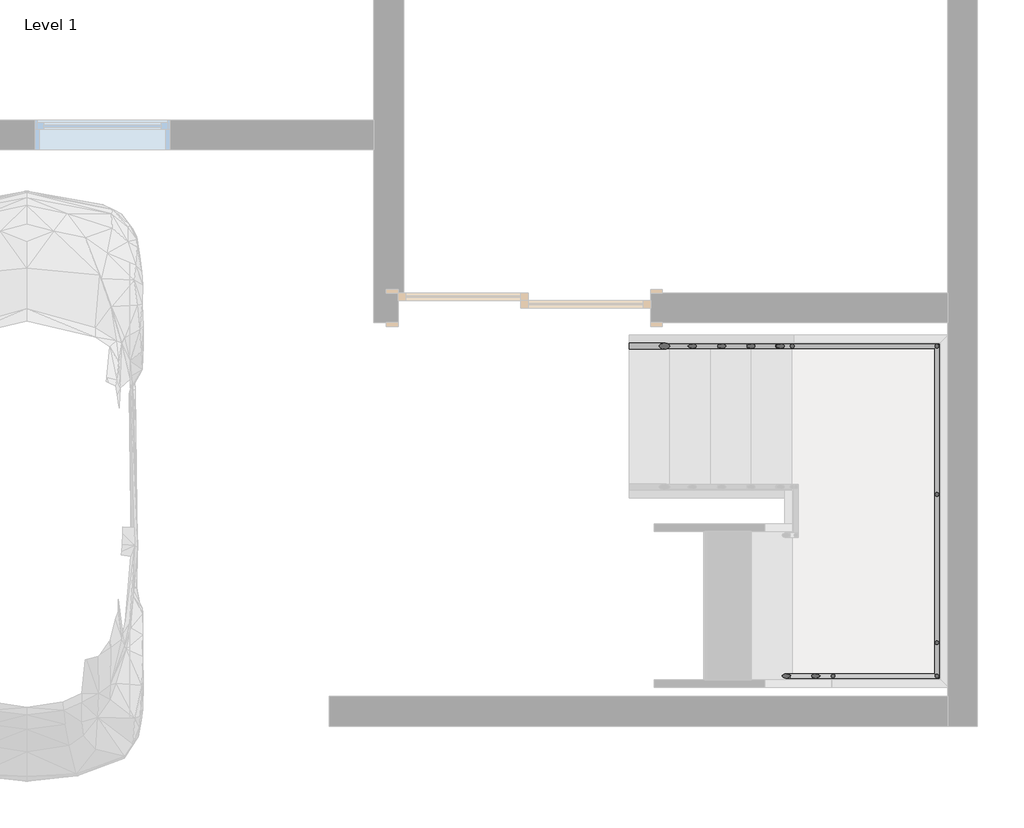
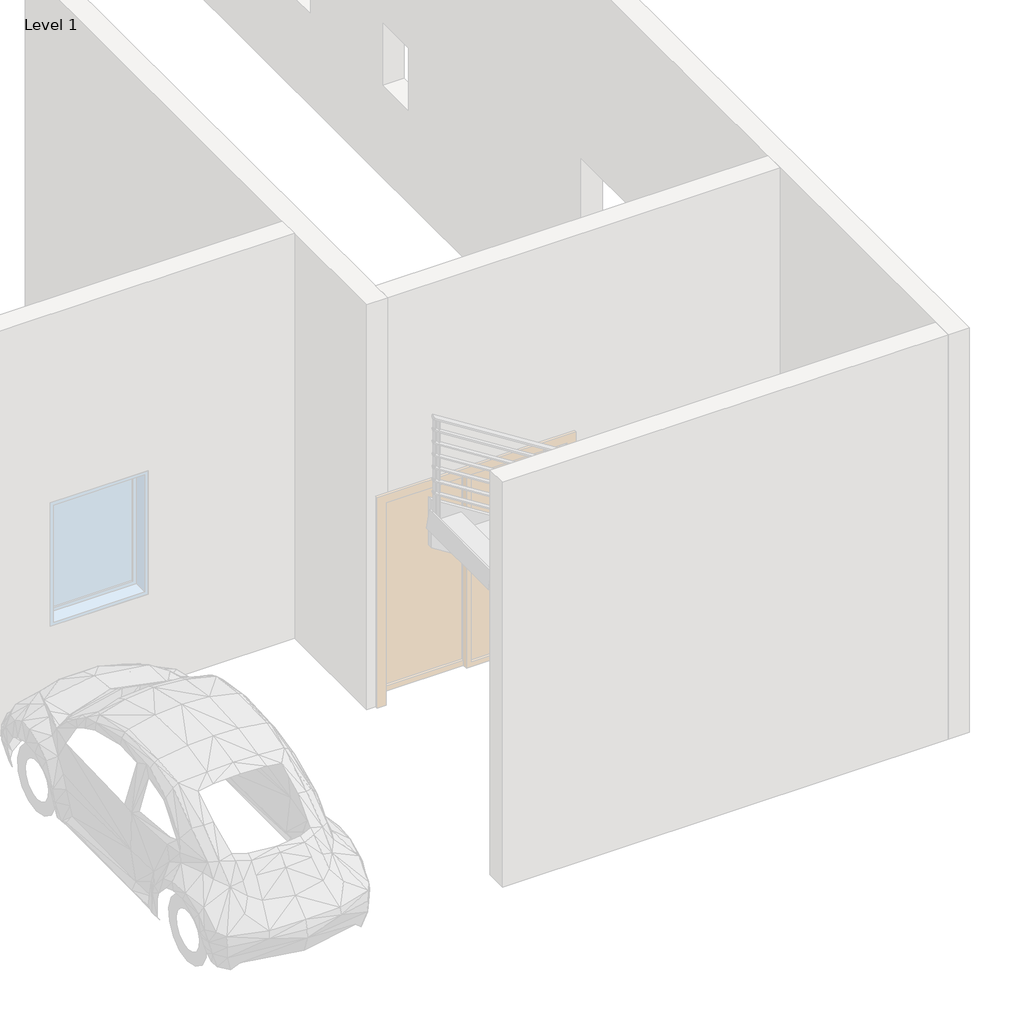
# One storey, part 3 of 4: 1 railing.
"""IFC4 building model written with IfcOpenShell, lengths in millimetres."""

from ifc_helpers import new_model, si_unit, point, frame, frame_2d, origin, place, context, project, spatial, circle_curve, ellipse_curve, trimmed, segment, composite_curve, outline, extrude, element, save
from ifc_brep_helpers import plane_surface, cylinder_surface, advanced_brep

model = new_model("IFC4")

# Units and contexts
model_context = context("Model", 3, world=origin())
ifc_project = project(units=[si_unit("LENGTHUNIT", "METRE", prefix="MILLI")], contexts=[model_context])

# Site, building, storey
site = spatial("IfcSite", under=ifc_project)
building = spatial("IfcBuilding", under=site)
storey = spatial("IfcBuildingStorey", under=building, Name="Level 1", Elevation=0.0)

# Railing
placement = place(None, origin())
element("IfcRailing", 1, ObjectType="900mm Pipe", at=placement, inside=storey, context=model_context, shape_type="SolidModel", body=[
    advanced_brep(
    [(-3791.9701746, -1586.5632824, 1050.2491997), (-3791.9701746, -1546.5632824, 1050.2491997), (-2686.1767216, -1586.5632824, 1749.5652174), (-2686.1767216, -1546.5632824, 1749.5652174), (-1737.3443934, -1586.5632824, 1749.5652174), (-1697.3443934, -1546.5632824, 1749.5652174), (-1737.3443934, -3770.8148449, 1749.5652174), (-1697.3443934, -3810.8148449, 1749.5652174), (-2422.7636276, -3770.8148449, 1749.5652174), (-2422.7636276, -3810.8148449, 1749.5652174), (-5716.9701746, -3770.8148449, 3832.8578953), (-5716.9701746, -3810.8148449, 3832.8578953)],
    [
        (0, 1, ellipse_curve(frame((-3791.9701746, -1566.5632824, 1050.2491997), z_axis=(-1.0, 0.0, 0.0), x_axis=(0.0, 0.0, -1.0)), 23.6638438, 20.0)),
        (1, 0, ellipse_curve(frame((-3791.9701746, -1566.5632824, 1050.2491997), z_axis=(-1.0, 0.0, 0.0), x_axis=(0.0, 0.0, -1.0)), 23.6638438, 20.0)),
        (0, 2),
        (2, 3, ellipse_curve(frame((-2686.1767216, -1566.5632824, 1749.5652174), z_axis=(-0.9605132043335073, 0.0, -0.27823440531497545), x_axis=(0.27823440531497523, 0.0, -0.9605132043335074)), 20.822202, 20.0)),
        (3, 1),
        (3, 2, ellipse_curve(frame((-2686.1767216, -1566.5632824, 1749.5652174), z_axis=(-0.9605132043335073, 0.0, -0.27823440531497545), x_axis=(0.27823440531497523, 0.0, -0.9605132043335074)), 20.822202, 20.0)),
        (2, 4),
        (4, 5, ellipse_curve(frame((-1717.3443934, -1566.5632824, 1749.5652174), z_axis=(-0.7071067811865449, 0.70710678118655, 0.0), x_axis=(-0.7071067811865501, -0.7071067811865448, 0.0)), 28.2842712, 20.0)),
        (5, 3),
        (5, 4, ellipse_curve(frame((-1717.3443934, -1566.5632824, 1749.5652174), z_axis=(-0.7071067811865449, 0.70710678118655, 0.0), x_axis=(-0.7071067811865501, -0.7071067811865448, 0.0)), 28.2842712, 20.0)),
        (4, 6),
        (6, 7, ellipse_curve(frame((-1717.3443934, -3790.8148449, 1749.5652174), z_axis=(0.70710678118655, 0.7071067811865449, 0.0), x_axis=(-0.7071067811865448, 0.7071067811865502, 0.0)), 28.2842712, 20.0)),
        (7, 5),
        (7, 6, ellipse_curve(frame((-1717.3443934, -3790.8148449, 1749.5652174), z_axis=(0.70710678118655, 0.7071067811865449, 0.0), x_axis=(-0.7071067811865448, 0.7071067811865502, 0.0)), 28.2842712, 20.0)),
        (6, 8),
        (8, 9, ellipse_curve(frame((-2422.7636276, -3790.8148449, 1749.5652174), z_axis=(0.9605132043335072, 0.0, -0.27823440531497556), x_axis=(0.27823440531497595, 0.0, 0.9605132043335071)), 20.822202, 20.0)),
        (9, 7),
        (9, 8, ellipse_curve(frame((-2422.7636276, -3790.8148449, 1749.5652174), z_axis=(0.9605132043335072, 0.0, -0.27823440531497556), x_axis=(0.27823440531497595, 0.0, 0.9605132043335071)), 20.822202, 20.0)),
        (10, 11, ellipse_curve(frame((-5716.9701746, -3790.8148449, 3832.8578953), z_axis=(-1.0, 0.0, 0.0), x_axis=(0.0, 0.0, -1.0)), 23.6638438, 20.0)),
        (11, 10, ellipse_curve(frame((-5716.9701746, -3790.8148449, 3832.8578953), z_axis=(-1.0, 0.0, 0.0), x_axis=(0.0, 0.0, -1.0)), 23.6638438, 20.0)),
        (8, 10),
        (11, 9),
    ],
    [
        plane_surface(frame((-3791.9701746, -1566.5632824, 1073.9130435), z_axis=(-1.0, 0.0, 0.0), x_axis=(0.0, 1.0, 0.0))),
        cylinder_surface(frame((-3781.2802618, -1566.5632824, 1057.0096189), z_axis=(-0.8451712313980438, 0.0, -0.53449564040983), x_axis=(0.0, 1.0, 0.0)), 20.0),
        cylinder_surface(frame((-2691.9701746, -1566.5632824, 1749.5652174), z_axis=(-1.0, 0.0, 0.0), x_axis=(0.0, 1.0, 0.0)), 20.0),
        cylinder_surface(frame((-1717.3443934, -1566.5632824, 1749.5652174), z_axis=(0.0, 1.0, 0.0), x_axis=(1.0, 0.0, 0.0)), 20.0),
        cylinder_surface(frame((-1717.3443934, -3790.8148449, 1749.5652174), z_axis=(1.0, 0.0, 0.0), x_axis=(0.0, -1.0, 0.0)), 20.0),
        plane_surface(frame((-5716.9701746, -3790.8148449, 3856.5217391), z_axis=(-1.0, 0.0, 0.0), x_axis=(0.0, -1.0, 0.0))),
        cylinder_surface(frame((-2427.6600875, -3790.8148449, 1752.6617928), z_axis=(0.8451712313980437, 0.0, -0.5344956404098302), x_axis=(0.0, -1.0, 0.0)), 20.0),
    ],
    [
        (0, [[1, 2]]),
        (1, [[-1, 3, 4, 5]]),
        (1, [[-2, -5, 6, -3]]),
        (2, [[-4, 7, 8, 9]]),
        (2, [[-6, -9, 10, -7]]),
        (3, [[-8, 11, 12, 13]]),
        (3, [[-10, -13, 14, -11]]),
        (4, [[-12, 15, 16, 17]]),
        (4, [[-14, -17, 18, -15]]),
        (5, [[19, 20]]),
        (6, [[-16, 21, -20, 22]]),
        (6, [[-18, -22, -19, -21]]),
    ],
),
    advanced_brep(
    [(-3791.9701746, -1581.5632824, 931.1651606), (-3791.9701746, -1551.5632824, 931.1651606), (-2687.6250849, -1581.5632824, 1629.5652174), (-2687.6250849, -1551.5632824, 1629.5652174), (-1732.3443934, -1581.5632824, 1629.5652174), (-1702.3443934, -1551.5632824, 1629.5652174), (-1732.3443934, -3775.8148449, 1629.5652174), (-1702.3443934, -3805.8148449, 1629.5652174), (-2421.3152644, -3775.8148449, 1629.5652174), (-2421.3152644, -3805.8148449, 1629.5652174), (-5716.9701746, -3775.8148449, 3713.7738563), (-5716.9701746, -3805.8148449, 3713.7738563)],
    [
        (0, 1, ellipse_curve(frame((-3791.9701746, -1566.5632824, 931.1651606), z_axis=(-1.0, 0.0, 0.0), x_axis=(0.0, 0.0, -1.0)), 17.7478828, 15.0)),
        (1, 0, ellipse_curve(frame((-3791.9701746, -1566.5632824, 931.1651606), z_axis=(-1.0, 0.0, 0.0), x_axis=(0.0, 0.0, -1.0)), 17.7478828, 15.0)),
        (0, 2),
        (2, 3, ellipse_curve(frame((-2687.6250849, -1566.5632824, 1629.5652174), z_axis=(-0.9605132043335073, 0.0, -0.27823440531497545), x_axis=(0.2782344053149749, 0.0, -0.9605132043335074)), 15.6166515, 15.0)),
        (3, 1),
        (3, 2, ellipse_curve(frame((-2687.6250849, -1566.5632824, 1629.5652174), z_axis=(-0.9605132043335073, 0.0, -0.27823440531497545), x_axis=(0.2782344053149749, 0.0, -0.9605132043335074)), 15.6166515, 15.0)),
        (2, 4),
        (4, 5, ellipse_curve(frame((-1717.3443934, -1566.5632824, 1629.5652174), z_axis=(-0.7071067811865449, 0.70710678118655, 0.0), x_axis=(-0.7071067811865501, -0.7071067811865448, 0.0)), 21.2132034, 15.0)),
        (5, 3),
        (5, 4, ellipse_curve(frame((-1717.3443934, -1566.5632824, 1629.5652174), z_axis=(-0.7071067811865449, 0.70710678118655, 0.0), x_axis=(-0.7071067811865501, -0.7071067811865448, 0.0)), 21.2132034, 15.0)),
        (4, 6),
        (6, 7, ellipse_curve(frame((-1717.3443934, -3790.8148449, 1629.5652174), z_axis=(0.70710678118655, 0.7071067811865449, 0.0), x_axis=(-0.7071067811865448, 0.7071067811865502, 0.0)), 21.2132034, 15.0)),
        (7, 5),
        (7, 6, ellipse_curve(frame((-1717.3443934, -3790.8148449, 1629.5652174), z_axis=(0.70710678118655, 0.7071067811865449, 0.0), x_axis=(-0.7071067811865448, 0.7071067811865502, 0.0)), 21.2132034, 15.0)),
        (6, 8),
        (8, 9, ellipse_curve(frame((-2421.3152644, -3790.8148449, 1629.5652174), z_axis=(0.9605132043335072, 0.0, -0.2782344053149756), x_axis=(0.27823440531497595, 0.0, 0.9605132043335071)), 15.6166515, 15.0)),
        (9, 7),
        (9, 8, ellipse_curve(frame((-2421.3152644, -3790.8148449, 1629.5652174), z_axis=(0.9605132043335072, 0.0, -0.2782344053149756), x_axis=(0.27823440531497595, 0.0, 0.9605132043335071)), 15.6166515, 15.0)),
        (10, 11, ellipse_curve(frame((-5716.9701746, -3790.8148449, 3713.7738563), z_axis=(-1.0, 0.0, 0.0), x_axis=(0.0, 0.0, -1.0)), 17.7478828, 15.0)),
        (11, 10, ellipse_curve(frame((-5716.9701746, -3790.8148449, 3713.7738563), z_axis=(-1.0, 0.0, 0.0), x_axis=(0.0, 0.0, -1.0)), 17.7478828, 15.0)),
        (8, 10),
        (11, 9),
    ],
    [
        plane_surface(frame((-3791.9701746, -1566.5632824, 948.9130435), z_axis=(-1.0, 0.0, 0.0), x_axis=(0.0, 1.0, 0.0))),
        cylinder_surface(frame((-3783.95274, -1566.5632824, 936.235475), z_axis=(-0.845171231398044, 0.0, -0.5344956404098299), x_axis=(0.0, 1.0, 0.0)), 15.0),
        cylinder_surface(frame((-2691.9701746, -1566.5632824, 1629.5652174), z_axis=(-1.0, 0.0, 0.0), x_axis=(0.0, 1.0, 0.0)), 15.0),
        cylinder_surface(frame((-1717.3443934, -1566.5632824, 1629.5652174), z_axis=(0.0, 1.0, 0.0), x_axis=(1.0, 0.0, 0.0)), 15.0),
        cylinder_surface(frame((-1717.3443934, -3790.8148449, 1629.5652174), z_axis=(1.0, 0.0, 0.0), x_axis=(0.0, -1.0, 0.0)), 15.0),
        plane_surface(frame((-5716.9701746, -3790.8148449, 3731.5217391), z_axis=(-1.0, 0.0, 0.0), x_axis=(0.0, -1.0, 0.0))),
        cylinder_surface(frame((-2424.9876092, -3790.8148449, 1631.8876489), z_axis=(0.8451712313980437, 0.0, -0.5344956404098302), x_axis=(0.0, -1.0, 0.0)), 15.0),
    ],
    [
        (0, [[1, 2]]),
        (1, [[-1, 3, 4, 5]]),
        (1, [[-2, -5, 6, -3]]),
        (2, [[-4, 7, 8, 9]]),
        (2, [[-6, -9, 10, -7]]),
        (3, [[-8, 11, 12, 13]]),
        (3, [[-10, -13, 14, -11]]),
        (4, [[-12, 15, 16, 17]]),
        (4, [[-14, -17, 18, -15]]),
        (5, [[19, 20]]),
        (6, [[-16, 21, -20, 22]]),
        (6, [[-18, -22, -19, -21]]),
    ],
),
    advanced_brep(
    [(-3791.9701746, -1581.5632824, 806.1651606), (-3791.9701746, -1551.5632824, 806.1651606), (-2687.6250849, -1581.5632824, 1504.5652174), (-2687.6250849, -1551.5632824, 1504.5652174), (-1732.3443934, -1581.5632824, 1504.5652174), (-1702.3443934, -1551.5632824, 1504.5652174), (-1732.3443934, -3775.8148449, 1504.5652174), (-1702.3443934, -3805.8148449, 1504.5652174), (-2421.3152644, -3775.8148449, 1504.5652174), (-2421.3152644, -3805.8148449, 1504.5652174), (-5716.9701746, -3775.8148449, 3588.7738563), (-5716.9701746, -3805.8148449, 3588.7738563)],
    [
        (0, 1, ellipse_curve(frame((-3791.9701746, -1566.5632824, 806.1651606), z_axis=(-1.0, 0.0, 0.0), x_axis=(0.0, 0.0, -1.0)), 17.7478828, 15.0)),
        (1, 0, ellipse_curve(frame((-3791.9701746, -1566.5632824, 806.1651606), z_axis=(-1.0, 0.0, 0.0), x_axis=(0.0, 0.0, -1.0)), 17.7478828, 15.0)),
        (0, 2),
        (2, 3, ellipse_curve(frame((-2687.6250849, -1566.5632824, 1504.5652174), z_axis=(-0.9605132043335073, 0.0, -0.27823440531497545), x_axis=(0.2782344053149749, 0.0, -0.9605132043335074)), 15.6166515, 15.0)),
        (3, 1),
        (3, 2, ellipse_curve(frame((-2687.6250849, -1566.5632824, 1504.5652174), z_axis=(-0.9605132043335073, 0.0, -0.27823440531497545), x_axis=(0.2782344053149749, 0.0, -0.9605132043335074)), 15.6166515, 15.0)),
        (2, 4),
        (4, 5, ellipse_curve(frame((-1717.3443934, -1566.5632824, 1504.5652174), z_axis=(-0.7071067811865449, 0.70710678118655, 0.0), x_axis=(-0.7071067811865501, -0.7071067811865448, 0.0)), 21.2132034, 15.0)),
        (5, 3),
        (5, 4, ellipse_curve(frame((-1717.3443934, -1566.5632824, 1504.5652174), z_axis=(-0.7071067811865449, 0.70710678118655, 0.0), x_axis=(-0.7071067811865501, -0.7071067811865448, 0.0)), 21.2132034, 15.0)),
        (4, 6),
        (6, 7, ellipse_curve(frame((-1717.3443934, -3790.8148449, 1504.5652174), z_axis=(0.70710678118655, 0.7071067811865449, 0.0), x_axis=(-0.7071067811865448, 0.7071067811865502, 0.0)), 21.2132034, 15.0)),
        (7, 5),
        (7, 6, ellipse_curve(frame((-1717.3443934, -3790.8148449, 1504.5652174), z_axis=(0.70710678118655, 0.7071067811865449, 0.0), x_axis=(-0.7071067811865448, 0.7071067811865502, 0.0)), 21.2132034, 15.0)),
        (6, 8),
        (8, 9, ellipse_curve(frame((-2421.3152644, -3790.8148449, 1504.5652174), z_axis=(0.9605132043335072, 0.0, -0.2782344053149756), x_axis=(0.27823440531497595, 0.0, 0.9605132043335071)), 15.6166515, 15.0)),
        (9, 7),
        (9, 8, ellipse_curve(frame((-2421.3152644, -3790.8148449, 1504.5652174), z_axis=(0.9605132043335072, 0.0, -0.2782344053149756), x_axis=(0.27823440531497595, 0.0, 0.9605132043335071)), 15.6166515, 15.0)),
        (10, 11, ellipse_curve(frame((-5716.9701746, -3790.8148449, 3588.7738563), z_axis=(-1.0, 0.0, 0.0), x_axis=(0.0, 0.0, -1.0)), 17.7478828, 15.0)),
        (11, 10, ellipse_curve(frame((-5716.9701746, -3790.8148449, 3588.7738563), z_axis=(-1.0, 0.0, 0.0), x_axis=(0.0, 0.0, -1.0)), 17.7478828, 15.0)),
        (8, 10),
        (11, 9),
    ],
    [
        plane_surface(frame((-3791.9701746, -1566.5632824, 823.9130435), z_axis=(-1.0, 0.0, 0.0), x_axis=(0.0, 1.0, 0.0))),
        cylinder_surface(frame((-3783.95274, -1566.5632824, 811.235475), z_axis=(-0.845171231398044, 0.0, -0.5344956404098299), x_axis=(0.0, 1.0, 0.0)), 15.0),
        cylinder_surface(frame((-2691.9701746, -1566.5632824, 1504.5652174), z_axis=(-1.0, 0.0, 0.0), x_axis=(0.0, 1.0, 0.0)), 15.0),
        cylinder_surface(frame((-1717.3443934, -1566.5632824, 1504.5652174), z_axis=(0.0, 1.0, 0.0), x_axis=(1.0, 0.0, 0.0)), 15.0),
        cylinder_surface(frame((-1717.3443934, -3790.8148449, 1504.5652174), z_axis=(1.0, 0.0, 0.0), x_axis=(0.0, -1.0, 0.0)), 15.0),
        plane_surface(frame((-5716.9701746, -3790.8148449, 3606.5217391), z_axis=(-1.0, 0.0, 0.0), x_axis=(0.0, -1.0, 0.0))),
        cylinder_surface(frame((-2424.9876092, -3790.8148449, 1506.8876489), z_axis=(0.8451712313980437, 0.0, -0.5344956404098302), x_axis=(0.0, -1.0, 0.0)), 15.0),
    ],
    [
        (0, [[1, 2]]),
        (1, [[-1, 3, 4, 5]]),
        (1, [[-2, -5, 6, -3]]),
        (2, [[-4, 7, 8, 9]]),
        (2, [[-6, -9, 10, -7]]),
        (3, [[-8, 11, 12, 13]]),
        (3, [[-10, -13, 14, -11]]),
        (4, [[-12, 15, 16, 17]]),
        (4, [[-14, -17, 18, -15]]),
        (5, [[19, 20]]),
        (6, [[-16, 21, -20, 22]]),
        (6, [[-18, -22, -19, -21]]),
    ],
),
    advanced_brep(
    [(-3791.9701746, -1581.5632824, 681.1651606), (-3791.9701746, -1551.5632824, 681.1651606), (-2687.6250849, -1581.5632824, 1379.5652174), (-2687.6250849, -1551.5632824, 1379.5652174), (-1732.3443934, -1581.5632824, 1379.5652174), (-1702.3443934, -1551.5632824, 1379.5652174), (-1732.3443934, -3775.8148449, 1379.5652174), (-1702.3443934, -3805.8148449, 1379.5652174), (-2421.3152644, -3775.8148449, 1379.5652174), (-2421.3152644, -3805.8148449, 1379.5652174), (-5716.9701746, -3775.8148449, 3463.7738563), (-5716.9701746, -3805.8148449, 3463.7738563)],
    [
        (0, 1, ellipse_curve(frame((-3791.9701746, -1566.5632824, 681.1651606), z_axis=(-1.0, 0.0, 0.0), x_axis=(0.0, 0.0, -1.0)), 17.7478828, 15.0)),
        (1, 0, ellipse_curve(frame((-3791.9701746, -1566.5632824, 681.1651606), z_axis=(-1.0, 0.0, 0.0), x_axis=(0.0, 0.0, -1.0)), 17.7478828, 15.0)),
        (0, 2),
        (2, 3, ellipse_curve(frame((-2687.6250849, -1566.5632824, 1379.5652174), z_axis=(-0.9605132043335073, 0.0, -0.27823440531497545), x_axis=(0.2782344053149749, 0.0, -0.9605132043335074)), 15.6166515, 15.0)),
        (3, 1),
        (3, 2, ellipse_curve(frame((-2687.6250849, -1566.5632824, 1379.5652174), z_axis=(-0.9605132043335073, 0.0, -0.27823440531497545), x_axis=(0.2782344053149749, 0.0, -0.9605132043335074)), 15.6166515, 15.0)),
        (2, 4),
        (4, 5, ellipse_curve(frame((-1717.3443934, -1566.5632824, 1379.5652174), z_axis=(-0.7071067811865449, 0.70710678118655, 0.0), x_axis=(-0.7071067811865501, -0.7071067811865448, 0.0)), 21.2132034, 15.0)),
        (5, 3),
        (5, 4, ellipse_curve(frame((-1717.3443934, -1566.5632824, 1379.5652174), z_axis=(-0.7071067811865449, 0.70710678118655, 0.0), x_axis=(-0.7071067811865501, -0.7071067811865448, 0.0)), 21.2132034, 15.0)),
        (4, 6),
        (6, 7, ellipse_curve(frame((-1717.3443934, -3790.8148449, 1379.5652174), z_axis=(0.70710678118655, 0.7071067811865449, 0.0), x_axis=(-0.7071067811865448, 0.7071067811865502, 0.0)), 21.2132034, 15.0)),
        (7, 5),
        (7, 6, ellipse_curve(frame((-1717.3443934, -3790.8148449, 1379.5652174), z_axis=(0.70710678118655, 0.7071067811865449, 0.0), x_axis=(-0.7071067811865448, 0.7071067811865502, 0.0)), 21.2132034, 15.0)),
        (6, 8),
        (8, 9, ellipse_curve(frame((-2421.3152644, -3790.8148449, 1379.5652174), z_axis=(0.9605132043335072, 0.0, -0.27823440531497556), x_axis=(0.27823440531497606, 0.0, 0.9605132043335073)), 15.6166515, 15.0)),
        (9, 7),
        (9, 8, ellipse_curve(frame((-2421.3152644, -3790.8148449, 1379.5652174), z_axis=(0.9605132043335072, 0.0, -0.27823440531497556), x_axis=(0.27823440531497606, 0.0, 0.9605132043335073)), 15.6166515, 15.0)),
        (10, 11, ellipse_curve(frame((-5716.9701746, -3790.8148449, 3463.7738563), z_axis=(-1.0, 0.0, 0.0), x_axis=(0.0, 0.0, -1.0)), 17.7478828, 15.0)),
        (11, 10, ellipse_curve(frame((-5716.9701746, -3790.8148449, 3463.7738563), z_axis=(-1.0, 0.0, 0.0), x_axis=(0.0, 0.0, -1.0)), 17.7478828, 15.0)),
        (8, 10),
        (11, 9),
    ],
    [
        plane_surface(frame((-3791.9701746, -1566.5632824, 698.9130435), z_axis=(-1.0, 0.0, 0.0), x_axis=(0.0, 1.0, 0.0))),
        cylinder_surface(frame((-3783.95274, -1566.5632824, 686.235475), z_axis=(-0.845171231398044, 0.0, -0.5344956404098299), x_axis=(0.0, 1.0, 0.0)), 15.0),
        cylinder_surface(frame((-2691.9701746, -1566.5632824, 1379.5652174), z_axis=(-1.0, 0.0, 0.0), x_axis=(0.0, 1.0, 0.0)), 15.0),
        cylinder_surface(frame((-1717.3443934, -1566.5632824, 1379.5652174), z_axis=(0.0, 1.0, 0.0), x_axis=(1.0, 0.0, 0.0)), 15.0),
        cylinder_surface(frame((-1717.3443934, -3790.8148449, 1379.5652174), z_axis=(1.0, 0.0, 0.0), x_axis=(0.0, -1.0, 0.0)), 15.0),
        plane_surface(frame((-5716.9701746, -3790.8148449, 3481.5217391), z_axis=(-1.0, 0.0, 0.0), x_axis=(0.0, -1.0, 0.0))),
        cylinder_surface(frame((-2424.9876092, -3790.8148449, 1381.8876489), z_axis=(0.8451712313980437, 0.0, -0.5344956404098301), x_axis=(0.0, -1.0, 0.0)), 15.0),
    ],
    [
        (0, [[1, 2]]),
        (1, [[-1, 3, 4, 5]]),
        (1, [[-2, -5, 6, -3]]),
        (2, [[-4, 7, 8, 9]]),
        (2, [[-6, -9, 10, -7]]),
        (3, [[-8, 11, 12, 13]]),
        (3, [[-10, -13, 14, -11]]),
        (4, [[-12, 15, 16, 17]]),
        (4, [[-14, -17, 18, -15]]),
        (5, [[19, 20]]),
        (6, [[-16, 21, -20, 22]]),
        (6, [[-18, -22, -19, -21]]),
    ],
),
    advanced_brep(
    [(-3791.9701746, -1581.5632824, 556.1651606), (-3791.9701746, -1551.5632824, 556.1651606), (-2687.6250849, -1581.5632824, 1254.5652174), (-2687.6250849, -1551.5632824, 1254.5652174), (-1732.3443934, -1581.5632824, 1254.5652174), (-1702.3443934, -1551.5632824, 1254.5652174), (-1732.3443934, -3775.8148449, 1254.5652174), (-1702.3443934, -3805.8148449, 1254.5652174), (-2421.3152644, -3775.8148449, 1254.5652174), (-2421.3152644, -3805.8148449, 1254.5652174), (-5716.9701746, -3775.8148449, 3338.7738563), (-5716.9701746, -3805.8148449, 3338.7738563)],
    [
        (0, 1, ellipse_curve(frame((-3791.9701746, -1566.5632824, 556.1651606), z_axis=(-1.0, 0.0, 0.0), x_axis=(0.0, 0.0, -1.0)), 17.7478828, 15.0)),
        (1, 0, ellipse_curve(frame((-3791.9701746, -1566.5632824, 556.1651606), z_axis=(-1.0, 0.0, 0.0), x_axis=(0.0, 0.0, -1.0)), 17.7478828, 15.0)),
        (0, 2),
        (2, 3, ellipse_curve(frame((-2687.6250849, -1566.5632824, 1254.5652174), z_axis=(-0.9605132043335073, 0.0, -0.27823440531497545), x_axis=(0.2782344053149749, 0.0, -0.9605132043335074)), 15.6166515, 15.0)),
        (3, 1),
        (3, 2, ellipse_curve(frame((-2687.6250849, -1566.5632824, 1254.5652174), z_axis=(-0.9605132043335073, 0.0, -0.27823440531497545), x_axis=(0.2782344053149749, 0.0, -0.9605132043335074)), 15.6166515, 15.0)),
        (2, 4),
        (4, 5, ellipse_curve(frame((-1717.3443934, -1566.5632824, 1254.5652174), z_axis=(-0.7071067811865449, 0.70710678118655, 0.0), x_axis=(-0.7071067811865501, -0.7071067811865448, 0.0)), 21.2132034, 15.0)),
        (5, 3),
        (5, 4, ellipse_curve(frame((-1717.3443934, -1566.5632824, 1254.5652174), z_axis=(-0.7071067811865449, 0.70710678118655, 0.0), x_axis=(-0.7071067811865501, -0.7071067811865448, 0.0)), 21.2132034, 15.0)),
        (4, 6),
        (6, 7, ellipse_curve(frame((-1717.3443934, -3790.8148449, 1254.5652174), z_axis=(0.70710678118655, 0.7071067811865449, 0.0), x_axis=(-0.7071067811865448, 0.7071067811865502, 0.0)), 21.2132034, 15.0)),
        (7, 5),
        (7, 6, ellipse_curve(frame((-1717.3443934, -3790.8148449, 1254.5652174), z_axis=(0.70710678118655, 0.7071067811865449, 0.0), x_axis=(-0.7071067811865448, 0.7071067811865502, 0.0)), 21.2132034, 15.0)),
        (6, 8),
        (8, 9, ellipse_curve(frame((-2421.3152644, -3790.8148449, 1254.5652174), z_axis=(0.9605132043335072, 0.0, -0.2782344053149756), x_axis=(0.27823440531497595, 0.0, 0.9605132043335071)), 15.6166515, 15.0)),
        (9, 7),
        (9, 8, ellipse_curve(frame((-2421.3152644, -3790.8148449, 1254.5652174), z_axis=(0.9605132043335072, 0.0, -0.2782344053149756), x_axis=(0.27823440531497595, 0.0, 0.9605132043335071)), 15.6166515, 15.0)),
        (10, 11, ellipse_curve(frame((-5716.9701746, -3790.8148449, 3338.7738563), z_axis=(-1.0, 0.0, 0.0), x_axis=(0.0, 0.0, -1.0)), 17.7478828, 15.0)),
        (11, 10, ellipse_curve(frame((-5716.9701746, -3790.8148449, 3338.7738563), z_axis=(-1.0, 0.0, 0.0), x_axis=(0.0, 0.0, -1.0)), 17.7478828, 15.0)),
        (8, 10),
        (11, 9),
    ],
    [
        plane_surface(frame((-3791.9701746, -1566.5632824, 573.9130435), z_axis=(-1.0, 0.0, 0.0), x_axis=(0.0, 1.0, 0.0))),
        cylinder_surface(frame((-3783.95274, -1566.5632824, 561.235475), z_axis=(-0.845171231398044, 0.0, -0.5344956404098299), x_axis=(0.0, 1.0, 0.0)), 15.0),
        cylinder_surface(frame((-2691.9701746, -1566.5632824, 1254.5652174), z_axis=(-1.0, 0.0, 0.0), x_axis=(0.0, 1.0, 0.0)), 15.0),
        cylinder_surface(frame((-1717.3443934, -1566.5632824, 1254.5652174), z_axis=(0.0, 1.0, 0.0), x_axis=(1.0, 0.0, 0.0)), 15.0),
        cylinder_surface(frame((-1717.3443934, -3790.8148449, 1254.5652174), z_axis=(1.0, 0.0, 0.0), x_axis=(0.0, -1.0, 0.0)), 15.0),
        plane_surface(frame((-5716.9701746, -3790.8148449, 3356.5217391), z_axis=(-1.0, 0.0, 0.0), x_axis=(0.0, -1.0, 0.0))),
        cylinder_surface(frame((-2424.9876092, -3790.8148449, 1256.8876489), z_axis=(0.8451712313980437, 0.0, -0.5344956404098302), x_axis=(0.0, -1.0, 0.0)), 15.0),
    ],
    [
        (0, [[1, 2]]),
        (1, [[-1, 3, 4, 5]]),
        (1, [[-2, -5, 6, -3]]),
        (2, [[-4, 7, 8, 9]]),
        (2, [[-6, -9, 10, -7]]),
        (3, [[-8, 11, 12, 13]]),
        (3, [[-10, -13, 14, -11]]),
        (4, [[-12, 15, 16, 17]]),
        (4, [[-14, -17, 18, -15]]),
        (5, [[19, 20]]),
        (6, [[-16, 21, -20, 22]]),
        (6, [[-18, -22, -19, -21]]),
    ],
),
    advanced_brep(
    [(-3791.9701746, -1581.5632824, 431.1651606), (-3791.9701746, -1551.5632824, 431.1651606), (-2687.6250849, -1581.5632824, 1129.5652174), (-2687.6250849, -1551.5632824, 1129.5652174), (-1732.3443934, -1581.5632824, 1129.5652174), (-1702.3443934, -1551.5632824, 1129.5652174), (-1732.3443934, -3775.8148449, 1129.5652174), (-1702.3443934, -3805.8148449, 1129.5652174), (-2421.3152644, -3775.8148449, 1129.5652174), (-2421.3152644, -3805.8148449, 1129.5652174), (-5716.9701746, -3775.8148449, 3213.7738563), (-5716.9701746, -3805.8148449, 3213.7738563)],
    [
        (0, 1, ellipse_curve(frame((-3791.9701746, -1566.5632824, 431.1651606), z_axis=(-1.0, 0.0, 0.0), x_axis=(0.0, 0.0, -1.0)), 17.7478828, 15.0)),
        (1, 0, ellipse_curve(frame((-3791.9701746, -1566.5632824, 431.1651606), z_axis=(-1.0, 0.0, 0.0), x_axis=(0.0, 0.0, -1.0)), 17.7478828, 15.0)),
        (0, 2),
        (2, 3, ellipse_curve(frame((-2687.6250849, -1566.5632824, 1129.5652174), z_axis=(-0.9605132043335073, 0.0, -0.27823440531497545), x_axis=(0.2782344053149749, 0.0, -0.9605132043335074)), 15.6166515, 15.0)),
        (3, 1),
        (3, 2, ellipse_curve(frame((-2687.6250849, -1566.5632824, 1129.5652174), z_axis=(-0.9605132043335073, 0.0, -0.27823440531497545), x_axis=(0.2782344053149749, 0.0, -0.9605132043335074)), 15.6166515, 15.0)),
        (2, 4),
        (4, 5, ellipse_curve(frame((-1717.3443934, -1566.5632824, 1129.5652174), z_axis=(-0.7071067811865449, 0.70710678118655, 0.0), x_axis=(-0.7071067811865501, -0.7071067811865448, 0.0)), 21.2132034, 15.0)),
        (5, 3),
        (5, 4, ellipse_curve(frame((-1717.3443934, -1566.5632824, 1129.5652174), z_axis=(-0.7071067811865449, 0.70710678118655, 0.0), x_axis=(-0.7071067811865501, -0.7071067811865448, 0.0)), 21.2132034, 15.0)),
        (4, 6),
        (6, 7, ellipse_curve(frame((-1717.3443934, -3790.8148449, 1129.5652174), z_axis=(0.70710678118655, 0.7071067811865449, 0.0), x_axis=(-0.7071067811865448, 0.7071067811865502, 0.0)), 21.2132034, 15.0)),
        (7, 5),
        (7, 6, ellipse_curve(frame((-1717.3443934, -3790.8148449, 1129.5652174), z_axis=(0.70710678118655, 0.7071067811865449, 0.0), x_axis=(-0.7071067811865448, 0.7071067811865502, 0.0)), 21.2132034, 15.0)),
        (6, 8),
        (8, 9, ellipse_curve(frame((-2421.3152644, -3790.8148449, 1129.5652174), z_axis=(0.9605132043335072, 0.0, -0.2782344053149756), x_axis=(0.27823440531497595, 0.0, 0.9605132043335071)), 15.6166515, 15.0)),
        (9, 7),
        (9, 8, ellipse_curve(frame((-2421.3152644, -3790.8148449, 1129.5652174), z_axis=(0.9605132043335072, 0.0, -0.2782344053149756), x_axis=(0.27823440531497595, 0.0, 0.9605132043335071)), 15.6166515, 15.0)),
        (10, 11, ellipse_curve(frame((-5716.9701746, -3790.8148449, 3213.7738563), z_axis=(-1.0, 0.0, 0.0), x_axis=(0.0, 0.0, -1.0)), 17.7478828, 15.0)),
        (11, 10, ellipse_curve(frame((-5716.9701746, -3790.8148449, 3213.7738563), z_axis=(-1.0, 0.0, 0.0), x_axis=(0.0, 0.0, -1.0)), 17.7478828, 15.0)),
        (8, 10),
        (11, 9),
    ],
    [
        plane_surface(frame((-3791.9701746, -1566.5632824, 448.9130435), z_axis=(-1.0, 0.0, 0.0), x_axis=(0.0, 1.0, 0.0))),
        cylinder_surface(frame((-3783.95274, -1566.5632824, 436.235475), z_axis=(-0.845171231398044, 0.0, -0.5344956404098299), x_axis=(0.0, 1.0, 0.0)), 15.0),
        cylinder_surface(frame((-2691.9701746, -1566.5632824, 1129.5652174), z_axis=(-1.0, 0.0, 0.0), x_axis=(0.0, 1.0, 0.0)), 15.0),
        cylinder_surface(frame((-1717.3443934, -1566.5632824, 1129.5652174), z_axis=(0.0, 1.0, 0.0), x_axis=(1.0, 0.0, 0.0)), 15.0),
        cylinder_surface(frame((-1717.3443934, -3790.8148449, 1129.5652174), z_axis=(1.0, 0.0, 0.0), x_axis=(0.0, -1.0, 0.0)), 15.0),
        plane_surface(frame((-5716.9701746, -3790.8148449, 3231.5217391), z_axis=(-1.0, 0.0, 0.0), x_axis=(0.0, -1.0, 0.0))),
        cylinder_surface(frame((-2424.9876092, -3790.8148449, 1131.8876489), z_axis=(0.8451712313980437, 0.0, -0.5344956404098302), x_axis=(0.0, -1.0, 0.0)), 15.0),
    ],
    [
        (0, [[1, 2]]),
        (1, [[-1, 3, 4, 5]]),
        (1, [[-2, -5, 6, -3]]),
        (2, [[-4, 7, 8, 9]]),
        (2, [[-6, -9, 10, -7]]),
        (3, [[-8, 11, 12, 13]]),
        (3, [[-10, -13, 14, -11]]),
        (4, [[-12, 15, 16, 17]]),
        (4, [[-14, -17, 18, -15]]),
        (5, [[19, 20]]),
        (6, [[-16, 21, -20, 22]]),
        (6, [[-18, -22, -19, -21]]),
    ],
),
    advanced_brep(
    [(-3791.9701746, -1581.5632824, 306.1651606), (-3791.9701746, -1551.5632824, 306.1651606), (-2687.6250849, -1581.5632824, 1004.5652174), (-2687.6250849, -1551.5632824, 1004.5652174), (-1732.3443934, -1581.5632824, 1004.5652174), (-1702.3443934, -1551.5632824, 1004.5652174), (-1732.3443934, -3775.8148449, 1004.5652174), (-1702.3443934, -3805.8148449, 1004.5652174), (-2421.3152644, -3775.8148449, 1004.5652174), (-2421.3152644, -3805.8148449, 1004.5652174), (-5716.9701746, -3775.8148449, 3088.7738563), (-5716.9701746, -3805.8148449, 3088.7738563)],
    [
        (0, 1, ellipse_curve(frame((-3791.9701746, -1566.5632824, 306.1651606), z_axis=(-1.0, 0.0, 0.0), x_axis=(0.0, 0.0, -1.0)), 17.7478828, 15.0)),
        (1, 0, ellipse_curve(frame((-3791.9701746, -1566.5632824, 306.1651606), z_axis=(-1.0, 0.0, 0.0), x_axis=(0.0, 0.0, -1.0)), 17.7478828, 15.0)),
        (0, 2),
        (2, 3, ellipse_curve(frame((-2687.6250849, -1566.5632824, 1004.5652174), z_axis=(-0.9605132043335073, 0.0, -0.27823440531497545), x_axis=(0.2782344053149749, 0.0, -0.9605132043335074)), 15.6166515, 15.0)),
        (3, 1),
        (3, 2, ellipse_curve(frame((-2687.6250849, -1566.5632824, 1004.5652174), z_axis=(-0.9605132043335073, 0.0, -0.27823440531497545), x_axis=(0.2782344053149749, 0.0, -0.9605132043335074)), 15.6166515, 15.0)),
        (2, 4),
        (4, 5, ellipse_curve(frame((-1717.3443934, -1566.5632824, 1004.5652174), z_axis=(-0.7071067811865449, 0.70710678118655, 0.0), x_axis=(-0.7071067811865501, -0.7071067811865448, 0.0)), 21.2132034, 15.0)),
        (5, 3),
        (5, 4, ellipse_curve(frame((-1717.3443934, -1566.5632824, 1004.5652174), z_axis=(-0.7071067811865449, 0.70710678118655, 0.0), x_axis=(-0.7071067811865501, -0.7071067811865448, 0.0)), 21.2132034, 15.0)),
        (4, 6),
        (6, 7, ellipse_curve(frame((-1717.3443934, -3790.8148449, 1004.5652174), z_axis=(0.70710678118655, 0.7071067811865449, 0.0), x_axis=(-0.7071067811865448, 0.7071067811865502, 0.0)), 21.2132034, 15.0)),
        (7, 5),
        (7, 6, ellipse_curve(frame((-1717.3443934, -3790.8148449, 1004.5652174), z_axis=(0.70710678118655, 0.7071067811865449, 0.0), x_axis=(-0.7071067811865448, 0.7071067811865502, 0.0)), 21.2132034, 15.0)),
        (6, 8),
        (8, 9, ellipse_curve(frame((-2421.3152644, -3790.8148449, 1004.5652174), z_axis=(0.9605132043335072, 0.0, -0.2782344053149756), x_axis=(0.27823440531497595, 0.0, 0.9605132043335071)), 15.6166515, 15.0)),
        (9, 7),
        (9, 8, ellipse_curve(frame((-2421.3152644, -3790.8148449, 1004.5652174), z_axis=(0.9605132043335072, 0.0, -0.2782344053149756), x_axis=(0.27823440531497595, 0.0, 0.9605132043335071)), 15.6166515, 15.0)),
        (10, 11, ellipse_curve(frame((-5716.9701746, -3790.8148449, 3088.7738563), z_axis=(-1.0, 0.0, 0.0), x_axis=(0.0, 0.0, -1.0)), 17.7478828, 15.0)),
        (11, 10, ellipse_curve(frame((-5716.9701746, -3790.8148449, 3088.7738563), z_axis=(-1.0, 0.0, 0.0), x_axis=(0.0, 0.0, -1.0)), 17.7478828, 15.0)),
        (8, 10),
        (11, 9),
    ],
    [
        plane_surface(frame((-3791.9701746, -1566.5632824, 323.9130435), z_axis=(-1.0, 0.0, 0.0), x_axis=(0.0, 1.0, 0.0))),
        cylinder_surface(frame((-3783.95274, -1566.5632824, 311.235475), z_axis=(-0.845171231398044, 0.0, -0.5344956404098299), x_axis=(0.0, 1.0, 0.0)), 15.0),
        cylinder_surface(frame((-2691.9701746, -1566.5632824, 1004.5652174), z_axis=(-1.0, 0.0, 0.0), x_axis=(0.0, 1.0, 0.0)), 15.0),
        cylinder_surface(frame((-1717.3443934, -1566.5632824, 1004.5652174), z_axis=(0.0, 1.0, 0.0), x_axis=(1.0, 0.0, 0.0)), 15.0),
        cylinder_surface(frame((-1717.3443934, -3790.8148449, 1004.5652174), z_axis=(1.0, 0.0, 0.0), x_axis=(0.0, -1.0, 0.0)), 15.0),
        plane_surface(frame((-5716.9701746, -3790.8148449, 3106.5217391), z_axis=(-1.0, 0.0, 0.0), x_axis=(0.0, -1.0, 0.0))),
        cylinder_surface(frame((-2424.9876092, -3790.8148449, 1006.8876489), z_axis=(0.8451712313980437, 0.0, -0.5344956404098302), x_axis=(0.0, -1.0, 0.0)), 15.0),
    ],
    [
        (0, [[1, 2]]),
        (1, [[-1, 3, 4, 5]]),
        (1, [[-2, -5, 6, -3]]),
        (2, [[-4, 7, 8, 9]]),
        (2, [[-6, -9, 10, -7]]),
        (3, [[-8, 11, 12, 13]]),
        (3, [[-10, -13, 14, -11]]),
        (4, [[-12, 15, 16, 17]]),
        (4, [[-14, -17, 18, -15]]),
        (5, [[19, 20]]),
        (6, [[-16, 21, -20, 22]]),
        (6, [[-18, -22, -19, -21]]),
    ],
),
    advanced_brep(
    [(-5416.9701746, -3803.3148449, 3619.4707314), (-5416.9701746, -3778.3148449, 3619.4707314), (-5416.9701746, -3778.3148449, 2608.6956522), (-5416.9701746, -3803.3148449, 2608.6956522)],
    [
        (0, 1, ellipse_curve(frame((-5416.9701746, -3790.8148449, 3619.4707314), z_axis=(-0.5344956404098286, 0.0, -0.8451712313980447), x_axis=(-0.8451712313980447, 0.0, 0.5344956404098286)), 14.7899024, 12.5)),
        (1, 2),
        (2, 3, circle_curve(frame((-5416.9701746, -3790.8148449, 2608.6956522), z_axis=(0.0, 0.0, 1.0), x_axis=(0.0, 1.0, 0.0)), 12.5)),
        (3, 0),
        (3, 2, circle_curve(frame((-5416.9701746, -3790.8148449, 2608.6956522), z_axis=(0.0, 0.0, 1.0), x_axis=(0.0, 1.0, 0.0)), 12.5)),
        (1, 0, ellipse_curve(frame((-5416.9701746, -3790.8148449, 3619.4707314), z_axis=(-0.5344956404098286, 0.0, -0.8451712313980447), x_axis=(-0.8451712313980447, 0.0, 0.5344956404098286)), 14.7899024, 12.5)),
    ],
    [
        cylinder_surface(frame((-5416.9701746, -3790.8148449, 2508.6956522), z_axis=(0.0, 0.0, 1.0), x_axis=(0.0, 1.0, 0.0)), 12.5),
        plane_surface(frame((-5441.9701746, -3765.8148449, 3635.2810081), z_axis=(0.5344956404098286, 0.0, 0.8451712313980447), x_axis=(0.0, -1.0, 0.0))),
        plane_surface(frame((-5391.9701746, -3765.8148449, 2608.6956522), z_axis=(0.0, 0.0, -1.0), x_axis=(0.0, -1.0, 0.0))),
    ],
    [
        (0, [[1, 2, 3, 4]]),
        (0, [[5, -2, 6, -4]]),
        (1, [[-6, -1]]),
        (2, [[-5, -3]]),
    ],
),
    advanced_brep(
    [(-4416.9701746, -3803.3148449, 2987.0596642), (-4416.9701746, -3778.3148449, 2987.0596642), (-4416.9701746, -3778.3148449, 2086.9565217), (-4416.9701746, -3803.3148449, 2086.9565217)],
    [
        (0, 1, ellipse_curve(frame((-4416.9701746, -3790.8148449, 2987.0596642), z_axis=(-0.5344956404098302, 0.0, -0.8451712313980437), x_axis=(-0.8451712313980437, 0.0, 0.53449564040983)), 14.7899024, 12.5)),
        (1, 2),
        (2, 3, circle_curve(frame((-4416.9701746, -3790.8148449, 2086.9565217), z_axis=(0.0, 0.0, 1.0), x_axis=(0.0, 1.0, 0.0)), 12.5)),
        (3, 0),
        (3, 2, circle_curve(frame((-4416.9701746, -3790.8148449, 2086.9565217), z_axis=(0.0, 0.0, 1.0), x_axis=(0.0, 1.0, 0.0)), 12.5)),
        (1, 0, ellipse_curve(frame((-4416.9701746, -3790.8148449, 2987.0596642), z_axis=(-0.5344956404098302, 0.0, -0.8451712313980437), x_axis=(-0.8451712313980437, 0.0, 0.53449564040983)), 14.7899024, 12.5)),
    ],
    [
        cylinder_surface(frame((-4416.9701746, -3790.8148449, 1986.9565217), z_axis=(0.0, 0.0, 1.0), x_axis=(0.0, 1.0, 0.0)), 12.5),
        plane_surface(frame((-4441.9701746, -3765.8148449, 3002.8699409), z_axis=(0.5344956404098302, 0.0, 0.8451712313980437), x_axis=(0.0, -1.0, 0.0))),
        plane_surface(frame((-4391.9701746, -3765.8148449, 2086.9565217), z_axis=(0.0, 0.0, -1.0), x_axis=(0.0, -1.0, 0.0))),
    ],
    [
        (0, [[1, 2, 3, 4]]),
        (0, [[5, -2, 6, -4]]),
        (1, [[-6, -1]]),
        (2, [[-5, -3]]),
    ],
),
    advanced_brep(
    [(-3416.9701746, -3803.3148449, 2354.648597), (-3416.9701746, -3778.3148449, 2354.648597), (-3416.9701746, -3778.3148449, 1391.3043478), (-3416.9701746, -3803.3148449, 1391.3043478)],
    [
        (0, 1, ellipse_curve(frame((-3416.9701746, -3790.8148449, 2354.648597), z_axis=(-0.5344956404098302, 0.0, -0.8451712313980437), x_axis=(-0.8451712313980437, 0.0, 0.53449564040983)), 14.7899024, 12.5)),
        (1, 2),
        (2, 3, circle_curve(frame((-3416.9701746, -3790.8148449, 1391.3043478), z_axis=(0.0, 0.0, 1.0), x_axis=(0.0, 1.0, 0.0)), 12.5)),
        (3, 0),
        (3, 2, circle_curve(frame((-3416.9701746, -3790.8148449, 1391.3043478), z_axis=(0.0, 0.0, 1.0), x_axis=(0.0, 1.0, 0.0)), 12.5)),
        (1, 0, ellipse_curve(frame((-3416.9701746, -3790.8148449, 2354.648597), z_axis=(-0.5344956404098302, 0.0, -0.8451712313980437), x_axis=(-0.8451712313980437, 0.0, 0.53449564040983)), 14.7899024, 12.5)),
    ],
    [
        cylinder_surface(frame((-3416.9701746, -3790.8148449, 1291.3043478), z_axis=(0.0, 0.0, 1.0), x_axis=(0.0, 1.0, 0.0)), 12.5),
        plane_surface(frame((-3441.9701746, -3765.8148449, 2370.4588737), z_axis=(0.5344956404098302, 0.0, 0.8451712313980437), x_axis=(0.0, -1.0, 0.0))),
        plane_surface(frame((-3391.9701746, -3765.8148449, 1391.3043478), z_axis=(0.0, 0.0, -1.0), x_axis=(0.0, -1.0, 0.0))),
    ],
    [
        (0, [[1, 2, 3, 4]]),
        (0, [[5, -2, 6, -4]]),
        (1, [[-6, -1]]),
        (2, [[-5, -3]]),
    ],
),
    extrude(outline(composite_curve([segment(trimmed(circle_curve(frame_2d((-1717.3443934, -3566.5632824)), 12.5), [point((-1729.8443934, -3566.5632824))], [point((-1704.8443934, -3566.5632824))], False, "CARTESIAN"), True, "CONTINUOUS"), segment(trimmed(circle_curve(frame_2d((-1717.3443934, -3566.5632824)), 12.5), [point((-1704.8443934, -3566.5632824))], [point((-1729.8443934, -3566.5632824))], False, "CARTESIAN"), True, "CONTINUOUS")], self_intersect=False)), frame((0.0, 0.0, 869.5652174), z_axis=(0.0, 0.0, 1.0), x_axis=(1.0, 0.0, 0.0)), (0.0, 0.0, 1.0), 860.0),
    extrude(outline(composite_curve([segment(trimmed(circle_curve(frame_2d((-1717.3443934, -2566.5632824)), 12.5), [point((-1729.8443934, -2566.5632824))], [point((-1704.8443934, -2566.5632824))], False, "CARTESIAN"), True, "CONTINUOUS"), segment(trimmed(circle_curve(frame_2d((-1717.3443934, -2566.5632824)), 12.5), [point((-1704.8443934, -2566.5632824))], [point((-1729.8443934, -2566.5632824))], False, "CARTESIAN"), True, "CONTINUOUS")], self_intersect=False)), frame((0.0, 0.0, 869.5652174), z_axis=(0.0, 0.0, 1.0), x_axis=(1.0, 0.0, 0.0)), (0.0, 0.0, 1.0), 860.0),
    advanced_brep(
    [(-2791.9701746, -1554.0632824, 1658.9964231), (-2791.9701746, -1579.0632824, 1658.9964231), (-2791.9701746, -1579.0632824, 695.6521739), (-2791.9701746, -1554.0632824, 695.6521739)],
    [
        (0, 1, ellipse_curve(frame((-2791.9701746, -1566.5632824, 1658.9964231), z_axis=(0.5344956404098302, 0.0, -0.8451712313980437), x_axis=(0.8451712313980437, 0.0, 0.53449564040983)), 14.7899024, 12.5)),
        (1, 2),
        (2, 3, circle_curve(frame((-2791.9701746, -1566.5632824, 695.6521739), z_axis=(0.0, 0.0, 1.0), x_axis=(0.0, -1.0, 0.0)), 12.5)),
        (3, 0),
        (3, 2, circle_curve(frame((-2791.9701746, -1566.5632824, 695.6521739), z_axis=(0.0, 0.0, 1.0), x_axis=(0.0, -1.0, 0.0)), 12.5)),
        (1, 0, ellipse_curve(frame((-2791.9701746, -1566.5632824, 1658.9964231), z_axis=(0.5344956404098302, 0.0, -0.8451712313980437), x_axis=(0.8451712313980437, 0.0, 0.53449564040983)), 14.7899024, 12.5)),
    ],
    [
        cylinder_surface(frame((-2791.9701746, -1566.5632824, 595.6521739), z_axis=(0.0, 0.0, 1.0), x_axis=(0.0, -1.0, 0.0)), 12.5),
        plane_surface(frame((-2766.9701746, -1591.5632824, 1674.8066998), z_axis=(-0.5344956404098302, 0.0, 0.8451712313980437), x_axis=(0.0, 1.0, 0.0))),
        plane_surface(frame((-2816.9701746, -1591.5632824, 695.6521739), z_axis=(0.0, 0.0, -1.0), x_axis=(0.0, 1.0, 0.0))),
    ],
    [
        (0, [[1, 2, 3, 4]]),
        (0, [[5, -2, 6, -4]]),
        (1, [[-6, -1]]),
        (2, [[-5, -3]]),
    ],
),
    advanced_brep(
    [(-2416.9701746, -3803.3148449, 1722.2375298), (-2416.9701746, -3778.3148449, 1722.2375298), (-2416.9701746, -3778.3148449, 869.5652174), (-2416.9701746, -3803.3148449, 869.5652174)],
    [
        (0, 1, ellipse_curve(frame((-2416.9701746, -3790.8148449, 1722.2375298), z_axis=(-0.5344956404098286, 0.0, -0.8451712313980447), x_axis=(-0.8451712313980447, 0.0, 0.5344956404098286)), 14.7899024, 12.5)),
        (1, 2),
        (2, 3, circle_curve(frame((-2416.9701746, -3790.8148449, 869.5652174), z_axis=(0.0, 0.0, 1.0), x_axis=(0.0, 1.0, 0.0)), 12.5)),
        (3, 0),
        (3, 2, circle_curve(frame((-2416.9701746, -3790.8148449, 869.5652174), z_axis=(0.0, 0.0, 1.0), x_axis=(0.0, 1.0, 0.0)), 12.5)),
        (1, 0, ellipse_curve(frame((-2416.9701746, -3790.8148449, 1722.2375298), z_axis=(-0.5344956404098286, 0.0, -0.8451712313980447), x_axis=(-0.8451712313980447, 0.0, 0.5344956404098286)), 14.7899024, 12.5)),
    ],
    [
        cylinder_surface(frame((-2416.9701746, -3790.8148449, 769.5652174), z_axis=(0.0, 0.0, 1.0), x_axis=(0.0, 1.0, 0.0)), 12.5),
        plane_surface(frame((-2441.9701746, -3765.8148449, 1738.0478065), z_axis=(0.5344956404098286, 0.0, 0.8451712313980447), x_axis=(0.0, -1.0, 0.0))),
        plane_surface(frame((-2391.9701746, -3765.8148449, 869.5652174), z_axis=(0.0, 0.0, -1.0), x_axis=(0.0, -1.0, 0.0))),
    ],
    [
        (0, [[1, 2, 3, 4]]),
        (0, [[5, -2, 6, -4]]),
        (1, [[-6, -1]]),
        (2, [[-5, -3]]),
    ],
),
    extrude(outline(composite_curve([segment(trimmed(circle_curve(frame_2d((-1717.3443934, -3790.8148449)), 12.5), [point((-1729.8443934, -3790.8148449))], [point((-1704.8443934, -3790.8148449))], False, "CARTESIAN"), True, "CONTINUOUS"), segment(trimmed(circle_curve(frame_2d((-1717.3443934, -3790.8148449)), 12.5), [point((-1704.8443934, -3790.8148449))], [point((-1729.8443934, -3790.8148449))], False, "CARTESIAN"), True, "CONTINUOUS")], self_intersect=False)), frame((0.0, 0.0, 869.5652174), z_axis=(0.0, 0.0, 1.0), x_axis=(1.0, 0.0, 0.0)), (0.0, 0.0, 1.0), 860.0),
    extrude(outline(composite_curve([segment(trimmed(circle_curve(frame_2d((-1717.3443934, -1566.5632824)), 12.5), [point((-1717.3443934, -1579.0632824))], [point((-1717.3443934, -1554.0632824))], False, "CARTESIAN"), True, "CONTINUOUS"), segment(trimmed(circle_curve(frame_2d((-1717.3443934, -1566.5632824)), 12.5), [point((-1717.3443934, -1554.0632824))], [point((-1717.3443934, -1579.0632824))], False, "CARTESIAN"), True, "CONTINUOUS")], self_intersect=False)), frame((0.0, 0.0, 869.5652174), z_axis=(0.0, 0.0, 1.0), x_axis=(1.0, 0.0, 0.0)), (0.0, 0.0, 1.0), 860.0),
    extrude(outline(composite_curve([segment(trimmed(circle_curve(frame_2d((-2691.9701746, -1566.5632824)), 12.5), [point((-2691.9701746, -1579.0632824))], [point((-2691.9701746, -1554.0632824))], False, "CARTESIAN"), True, "CONTINUOUS"), segment(trimmed(circle_curve(frame_2d((-2691.9701746, -1566.5632824)), 12.5), [point((-2691.9701746, -1554.0632824))], [point((-2691.9701746, -1579.0632824))], False, "CARTESIAN"), True, "CONTINUOUS")], self_intersect=False)), frame((0.0, 0.0, 869.5652174), z_axis=(0.0, 0.0, 1.0), x_axis=(1.0, 0.0, 0.0)), (0.0, 0.0, 1.0), 860.0),
    advanced_brep(
    [(-5704.4701746, -3803.3148449, 3801.2889132), (-5704.4701746, -3778.3148449, 3801.2889132), (-5704.4701746, -3778.3148449, 2782.6086957), (-5704.4701746, -3803.3148449, 2782.6086957)],
    [
        (0, 1, ellipse_curve(frame((-5704.4701746, -3790.8148449, 3801.2889132), z_axis=(-0.5344956404098302, 0.0, -0.8451712313980437), x_axis=(-0.8451712313980437, 0.0, 0.53449564040983)), 14.7899024, 12.5)),
        (1, 2),
        (2, 3, circle_curve(frame((-5704.4701746, -3790.8148449, 2782.6086957), z_axis=(0.0, 0.0, 1.0), x_axis=(0.0, 1.0, 0.0)), 12.5)),
        (3, 0),
        (3, 2, circle_curve(frame((-5704.4701746, -3790.8148449, 2782.6086957), z_axis=(0.0, 0.0, 1.0), x_axis=(0.0, 1.0, 0.0)), 12.5)),
        (1, 0, ellipse_curve(frame((-5704.4701746, -3790.8148449, 3801.2889132), z_axis=(-0.5344956404098302, 0.0, -0.8451712313980437), x_axis=(-0.8451712313980437, 0.0, 0.53449564040983)), 14.7899024, 12.5)),
    ],
    [
        cylinder_surface(frame((-5704.4701746, -3790.8148449, 2682.6086957), z_axis=(0.0, 0.0, 1.0), x_axis=(0.0, 1.0, 0.0)), 12.5),
        plane_surface(frame((-5729.4701746, -3765.8148449, 3817.0991899), z_axis=(0.5344956404098302, 0.0, 0.8451712313980437), x_axis=(0.0, -1.0, 0.0))),
        plane_surface(frame((-5679.4701746, -3765.8148449, 2782.6086957), z_axis=(0.0, 0.0, -1.0), x_axis=(0.0, -1.0, 0.0))),
    ],
    [
        (0, [[1, 2, 3, 4]]),
        (0, [[5, -2, 6, -4]]),
        (1, [[-6, -1]]),
        (2, [[-5, -3]]),
    ],
),
    advanced_brep(
    [(-3779.4701746, -1554.0632824, 1034.4904942), (-3779.4701746, -1579.0632824, 1034.4904942), (-3779.4701746, -1579.0632824, 173.9130435), (-3779.4701746, -1554.0632824, 173.9130435)],
    [
        (0, 1, ellipse_curve(frame((-3779.4701746, -1566.5632824, 1034.4904942), z_axis=(0.5344956404098302, 0.0, -0.8451712313980437), x_axis=(0.8451712313980437, 0.0, 0.53449564040983)), 14.7899024, 12.5)),
        (1, 2),
        (2, 3, circle_curve(frame((-3779.4701746, -1566.5632824, 173.9130435), z_axis=(0.0, 0.0, 1.0), x_axis=(0.0, -1.0, 0.0)), 12.5)),
        (3, 0),
        (3, 2, circle_curve(frame((-3779.4701746, -1566.5632824, 173.9130435), z_axis=(0.0, 0.0, 1.0), x_axis=(0.0, -1.0, 0.0)), 12.5)),
        (1, 0, ellipse_curve(frame((-3779.4701746, -1566.5632824, 1034.4904942), z_axis=(0.5344956404098302, 0.0, -0.8451712313980437), x_axis=(0.8451712313980437, 0.0, 0.53449564040983)), 14.7899024, 12.5)),
    ],
    [
        cylinder_surface(frame((-3779.4701746, -1566.5632824, 73.9130435), z_axis=(0.0, 0.0, 1.0), x_axis=(0.0, -1.0, 0.0)), 12.5),
        plane_surface(frame((-3754.4701746, -1591.5632824, 1050.3007709), z_axis=(-0.5344956404098302, 0.0, 0.8451712313980437), x_axis=(0.0, 1.0, 0.0))),
        plane_surface(frame((-3804.4701746, -1591.5632824, 173.9130435), z_axis=(0.0, 0.0, -1.0), x_axis=(0.0, 1.0, 0.0))),
    ],
    [
        (0, [[1, 2, 3, 4]]),
        (0, [[5, -2, 6, -4]]),
        (1, [[-6, -1]]),
        (2, [[-5, -3]]),
    ],
),
])

save(model, "model.ifc")

# Revit data of these elements
# Type "900mm Pipe"
#   built-in parameter 1008612 = 0.019685 (stored number, unit not read)
#   built-in parameter 1008611 = 0.0984252 (stored number, unit not read)
#   built-in parameter 1008609 = 6.56168 (stored number, unit not read)
#   built-in parameter 1008604 = 0.19685 (stored number, unit not read)
#   built-in parameter 1008603 = 0.164042 (stored number, unit not read)
#   Railing Height = 2' - 11.43307"
#   built-in parameter 1008630 = 2
#   built-in parameter 1008610 = 2
#   built-in parameter 1008605 = 1
#   built-in parameter 1008618 = M_Baluster - Round : 25mm
# Element 1 (IfcRailing, "900mm Pipe")
#   Phase Created = New Construction
